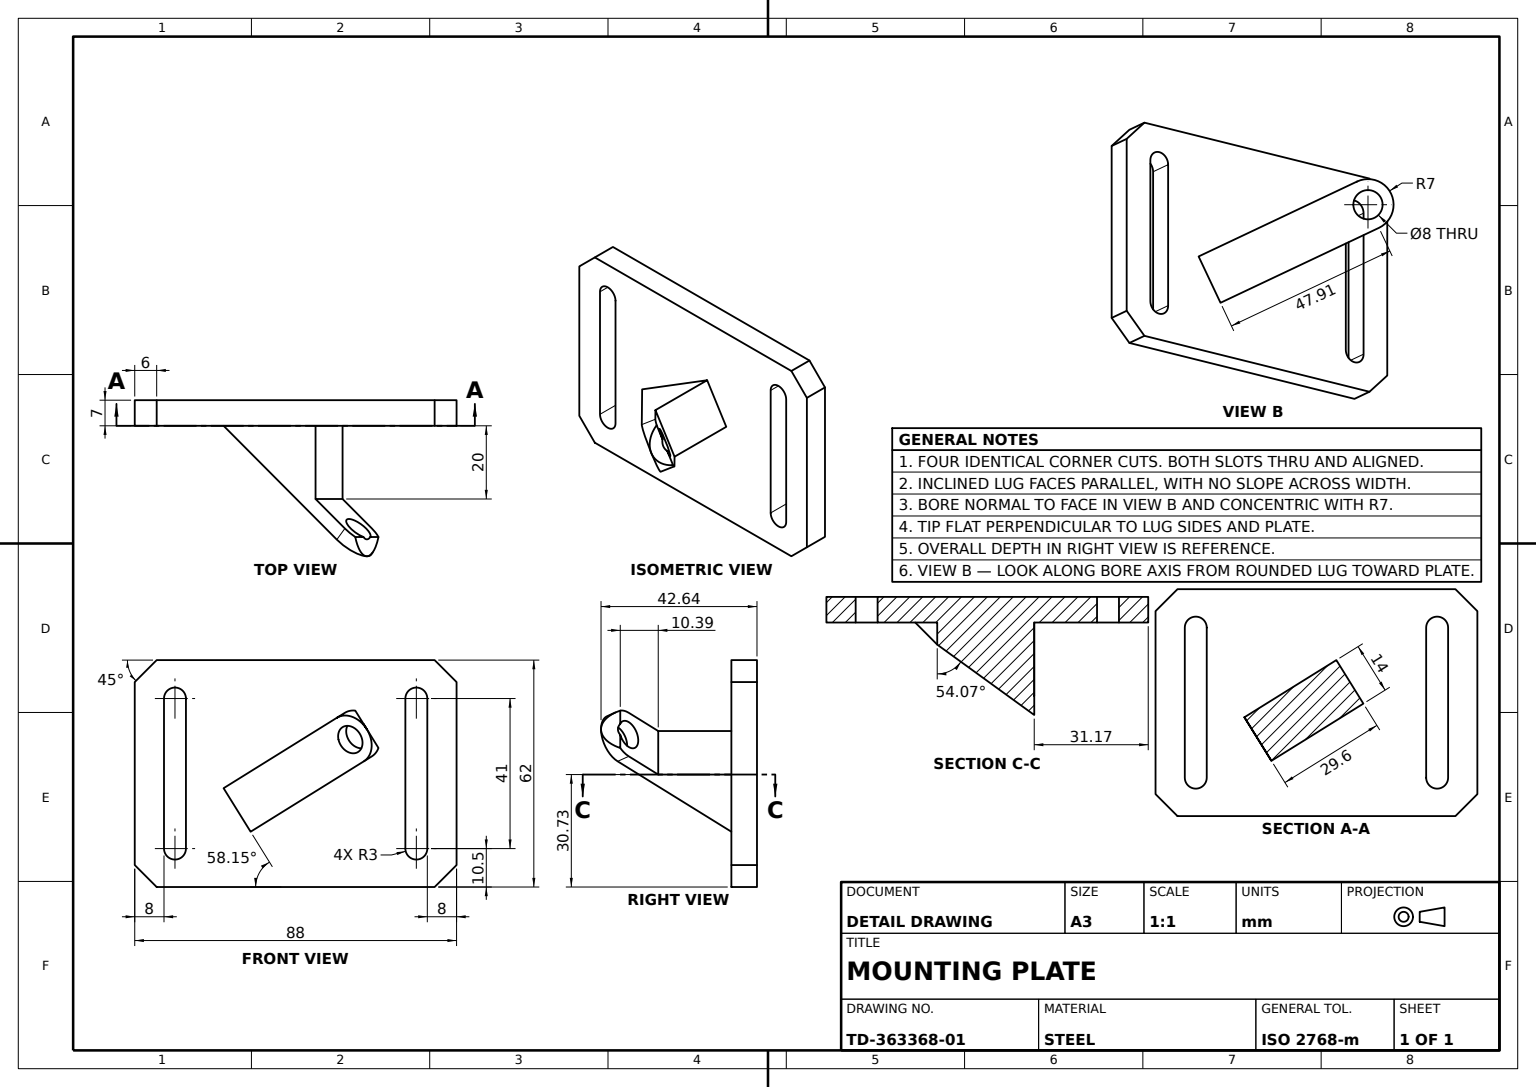
SolidWorks part; units mm, degrees
material "Plain Carbon Steel"
ref_plane "Front Plane" through (0, 0, 0) normal (0, 0, 1) x (1, 0, 0)
ref_plane "Top Plane" through (0, 0, 0) normal (0, 1, 0) x (1, 0, 0)
ref_plane "Right Plane" through (0, 0, 0) normal (1, 0, 0) x (0, 0, -1)
sketch "Base Plate Sketch" plane through (0, 0, 0) normal (0, 0, 1) x (1, 0, 0)
  line L0 (-44, 25) -> (-38, 31)
  line L1 (-38, 31) -> (38, 31)
  line L2 (-44, 25) -> (-44, -25)
  line L3 (-38, -31) -> (38, -31)
  line L4 (44, 25) -> (44, -25)
  line L5 (-44, 31) -> (44, -31) construction
  line L6 (-44, -31) -> (44, 31) construction
  line L7 (38, 31) -> (44, 25)
  line L8 (38, -31) -> (44, -25)
  line L9 (-44, -25) -> (-38, -31)
  line L10 (-33, 20.5) -> (-33, -20.5) construction
  line L11 (-30, 20.5) -> (-30, -20.5)
  line L12 (-36, 20.5) -> (-36, -20.5)
  line L13 (33, 20.5) -> (33, -20.5) construction
  line L16 (36, 20.5) -> (36, -20.5)
  line L17 (30, 20.5) -> (30, -20.5)
  arc A0 (-30, 20.5) -> (-36, 20.5) centre (-33, 20.5) ccw
  arc A1 (-36, -20.5) -> (-30, -20.5) centre (-33, -20.5) ccw
  arc A4 (36, 20.5) -> (30, 20.5) centre (33, 20.5) ccw
  arc A5 (30, -20.5) -> (36, -20.5) centre (33, -20.5) ccw
  point P0 (0, 0)
  point P16 (-33, 0)
  point P23 (33, 0)
  dimension "D1" = 88
  dimension "D2" = 62
  dimension "D3" = 6
  dimension "D4" = 45
  dimension "D5" = 6
  dimension "D6" = 45
  dimension "D7" = 6
  dimension "D8" = 45
  dimension "D9" = 6
  dimension "D10" = 45
  dimension "D11" = 8
  dimension "D12" = 8
  dimension "D13" = 6
  dimension "D14" = 6
  dimension "D15" = 41
  dimension "D16" = 41
  dimension "D17" = 10.5
  dimension "D18" = 10.5
extrude "Base Plate" add sketch "Base Plate Sketch" along normal blind 7
sketch "Block Axis Line" plane through (0, 0, 0) normal (0, 0, 1) x (1, 0, 0)
  line L0 (-33, -20.5) -> (33, 20.5) construction
ref_plane "Block Reference Plane" through (0, 0, 0) normal (0.5277, -0.8494, 0) x (0.8494, 0.5277, 0)
sketch "Angled Block Sketch" plane through (0, 0, 0) normal (0, 0, 1) x (1, 0, 0)
  line L0 (-19.705, -4.0002) -> (-12.3174, -15.8924)
  line L1 (-19.705, -4.0002) -> (15.7793, 18.043)
  line L2 (-12.3174, -15.8924) -> (23.1669, 6.1508)
  line L3 (15.7793, 18.043) -> (23.1669, 6.1508)
  line L4 (-33, -20.5) -> (33, 20.5) construction
  dimension "D1" = 20
  dimension "D2" = 14
  dimension "D3" = 35.4843
extrude "Angled Block" add sketch "Angled Block Sketch" along normal blind 50
sketch "Block Notch Sketch" plane through (0, 0, 0) normal (0.5277, -0.8494, 0) x (0.8494, 0.5277, 0)
  line L0 (-18.8491, 7) -> (22.9246, 42.6436)
  line L4 (10.7531, 7) -> (10.7531, 27)
  line L5 (15.4838, 7) -> (-18.8491, 7)
  line L8 (10.7531, 27) -> (22.9246, 37.3854)
  line L9 (22.9246, 37.3854) -> (22.9246, 42.6436)
  line L12 (-18.8491, 50) -> (-18.8491, 7)
  line L13 (-18.8491, 7) -> (22.9246, 7)
  line L14 (22.9246, 7) -> (22.9246, 50)
  line L15 (22.9246, 50) -> (-18.8491, 50)
  line L16 (-18.8491, 50) -> (-18.8491, 7)
  line L17 (-18.8491, 7) -> (22.9246, 7)
  line L18 (22.9246, 7) -> (22.9246, 50)
  line L19 (22.9246, 50) -> (-18.8491, 50)
  dimension "D1" = 20
  dimension "D2" = 4
  dimension "D3" = 16
  dimension "D4" = 34.3328
  dimension "D5" = 0
  dimension "D6" = 40.473
extrude "Block Notch Cut" cut sketch "Block Notch Sketch" against normal through all both and the other way through all contours L18 L19 L16 L0 | L17 L18 L8 L4 L5
sketch "Block Recess Sketch" plane through (-9.6817, -6.0144, 13.3579) normal (-0.5514, -0.3425, 0.7607) x (0.8343, -0.2264, 0.5027)
  line L0 (30.519, 33.9597) -> (39.3741, 23.116) construction
  line L1 (-12.0145, -0.7737) -> (30.519, 33.9597) construction
  line L2 (39.3741, 23.116) -> (-3.1593, -11.6174) construction
  line L7 (-12.0145, -0.7737) -> (-3.1593, -11.6174)
  line L8 (-3.1593, -11.6174) -> (39.3741, 23.116)
  line L9 (39.3741, 23.116) -> (30.519, 33.9597)
  line L10 (30.519, 33.9597) -> (-12.0145, -0.7737)
  line L11 (-12.0145, -0.7737) -> (-3.1593, -11.6174)
  line L12 (-3.1593, -11.6174) -> (39.3741, 23.116)
  line L13 (39.3741, 23.116) -> (30.519, 33.9597)
  line L14 (30.519, 33.9597) -> (-12.0145, -0.7737)
  circle A0 centre (29.5247, 24.1103) radius 7
  circle A1 centre (29.5247, 24.1103) radius 4
  line M9 (39.3741, 23.116) -> (30.519, 33.9597)
  line M10 (30.519, 33.9597) -> (-12.0145, -0.7737)
  dimension "D1" = 0
  dimension "D2" = 8
extrude "Block Recess Cut" cut sketch "Block Recess Sketch" against normal blind 13 and the other way through all contours A1 | A0 L12 M9 | A0 L13 M10
